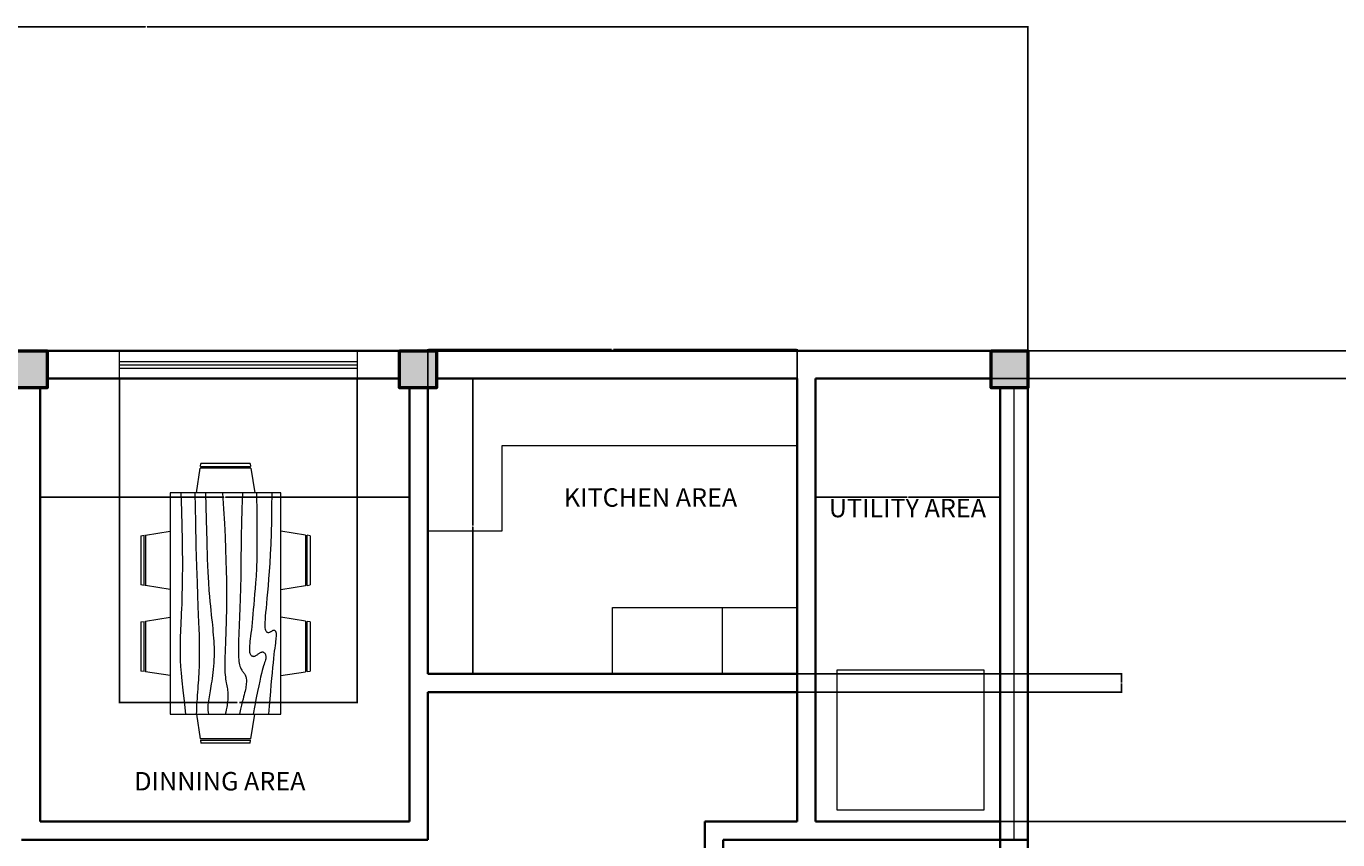
# Model space of a CAD drawing. Units: inches. Extents: x 369 to 4994, y 516 to 1297.
# Tile 3 of 9: x 722 to 1148, y 880 to 1144. Entities that reach past the tile are written whole.
import ezdxf

# ---------------------------------------------------------------- set-up
doc = ezdxf.new("R2010")
doc.units = ezdxf.units.IN
doc.header["$MEASUREMENT"] = 0
for name, color, linetype, lineweight in [('A-ANNO-DIMS', 2, 'Continuous', 18), ('A-AREA-IDEN', 7, 'Continuous', 18), ('A-COLS', 7, 'Continuous', 50), ('A-FLOR-CASE', 8, 'Continuous', 18), ('A-FURN', 8, 'Continuous', 18), ('A-GLAZ', 4, 'Continuous', 18), ('A-WALL', 7, 'Continuous', 35)]:
    doc.layers.add(name, color=color, linetype=linetype, lineweight=lineweight)
doc.layers.add('A-COLS-PATT', color=18, linetype='Continuous', lineweight=13, true_color=0x000000)
doc.styles.get("Standard").update_dxf_attribs({"font": 'arial.ttf'})
doc.dimstyles.get("Standard").update_dxf_attribs({"dimtxt": 0.18, "dimasz": 0.18, "dimexe": 0.18, "dimexo": 0.0625, "dimgap": 0.09, "dimtad": 0, "dimtih": 1, "dimtoh": 1, "dimdec": 4, "dimzin": 0, "dimdsep": 46, "dimtxsty": 'Standard', "dimcen": 0.09, "dimadec": 0, "dimazin": 0, "dimtfac": 1, "dimtdec": 4, "dimtofl": 0, "dimtmove": 0, "dimatfit": 3, "dimfxl": 1, "dimtolj": 1, "dimtzin": 0, "dimarcsym": 0})

# ---------------------------------------------------------------- blocks, each defined once
blk = doc.blocks.new('Dining Set - 36 x 72 in.')
for p, q in [((-22.2343, 26.00059), (-23.4847, 17.99762)), ((-22.2304, 26), (-5.7608, 26)), ((-22, 27.5), (-22.1562, 26.50042)), ((-5.8416, 26.5), (-22.1534, 26.5)), ((-22, 27.5), (-6, 27.5)), ((-5.8437, 26.49966), (-6, 27.5)), ((-4.5152, 17.99762), (-5.7655, 25.99926)), ((5.7657, 26.00059), (4.5153, 17.99762)), ((5.7696, 26), (22.2392, 26)), ((6, 27.5), (5.8438, 26.50042)), ((22.1584, 26.5), (5.8466, 26.5)), ((6, 27.5), (22, 27.5)), ((22.1563, 26.49966), (22, 27.5)), ((23.4848, 17.99762), (22.2345, 25.99926)), ((36, 18), (-36, 18)), ((-36, 18), (-36, -18)), ((36, -18), (36, 18)), ((-44.0006, 8.23428), (-35.9976, 9.48474)), ((44.0006, 8.23428), (35.9976, 9.48474)), ((-45.5, 8), (-44.5004, 8.15617)), ((-45.5, 8), (-45.5, -8)), ((-44.5, -8.15843), (-44.5, 8.15338)), ((-44, 8.23041), (-44, -8.23915)), ((44, 8.23041), (44, -8.23915)), ((44.5, -8.15843), (44.5, 8.15338)), ((45.5, 8), (44.5005, 8.15617)), ((45.5, 8), (45.5, -8)), ((-44.4997, -8.15631), (-45.5, -8)), ((-35.9976, -9.48476), (-43.9993, -8.2345)), ((35.9976, -9.48476), (43.9993, -8.2345)), ((44.4997, -8.15631), (45.5, -8)), ((-36, -18), (36, -18)), ((-22.2343, -26.0006), (-23.4847, -17.99762)), ((-4.5152, -17.99762), (-5.7655, -25.99928)), ((5.7657, -26.0006), (4.5153, -17.99762)), ((23.4848, -17.99762), (22.2345, -25.99928)), ((-22.2304, -26), (-5.7608, -26)), ((-22, -27.5), (-22.1562, -26.50044)), ((-5.8416, -26.5), (-22.1534, -26.5)), ((-22, -27.5), (-6, -27.5)), ((-5.8437, -26.49967), (-6, -27.5)), ((5.7696, -26), (22.2392, -26)), ((6, -27.5), (5.8438, -26.50044)), ((22.1584, -26.5), (5.8466, -26.5)), ((6, -27.5), (22, -27.5)), ((22.1563, -26.49967), (22, -27.5))]:
    blk.add_line(p, q)
for points in [[(-36, 15), (-31.1772, 14.97754), (-26.8079, 14.91406), (-22.8538, 14.81543), (-19.276, 14.6875), (-16.0362, 14.53613), (-13.0957, 14.36718), (-10.4159, 14.18652), (-7.9583, 14), (-5.6904, 13.81315), (-3.6035, 13.63021), (-1.6954, 13.45508), (0.0365, 13.29166), (1.5945, 13.14388), (2.9811, 13.01562), (4.1988, 12.9108), (5.25, 12.83333), (6.1393, 12.78613), (6.8802, 12.76823), (7.4883, 12.77767), (7.9792, 12.8125), (8.3685, 12.87077), (8.6719, 12.95052), (8.9049, 13.0498), (9.0833, 13.16666), (9.2205, 13.29899), (9.3216, 13.44401), (9.3895, 13.59879), (9.4271, 13.76041), (9.4373, 13.92594), (9.4232, 14.09245), (9.3875, 14.257), (9.3333, 14.41666), (9.2638, 14.56917), (9.1836, 14.71484), (9.0975, 14.85465), (9.0104, 14.98958), (8.9272, 15.1206), (8.8529, 15.2487), (8.7922, 15.37483), (8.75, 15.5), (8.7305, 15.62467), (8.7344, 15.74739), (8.7617, 15.86621), (8.8125, 15.97916), (8.8867, 16.08431), (8.9844, 16.17968), (9.1055, 16.26334), (9.25, 16.33333), (9.4189, 16.38802), (9.6172, 16.42708), (9.8506, 16.45052), (10.125, 16.45833), (10.4463, 16.45052), (10.8203, 16.42708), (11.2529, 16.38802), (11.75, 16.33333), (12.3184, 16.26318), (12.9694, 16.17838), (13.7151, 16.07991), (14.5677, 15.96875), (15.5395, 15.84586), (16.6426, 15.71224), (17.8893, 15.56884), (19.2917, 15.41666), (20.859, 15.25667), (22.5879, 15.08984), (24.4721, 14.91715), (26.5052, 14.73958), (28.6809, 14.5581), (30.9929, 14.3737), (33.4347, 14.18733), (36, 14)], [(-36, 10), (-28.9766, 10.14274), (-23.1725, 10.20442), (-18.4241, 10.19775), (-14.5677, 10.13541), (-11.4399, 10.03011), (-8.877, 9.89453), (-6.7154, 9.74137), (-4.7917, 9.58333), (-2.9698, 9.43082), (-1.2246, 9.28515), (0.4415, 9.14534), (2.026, 9.01041), (3.5266, 8.87939), (4.9408, 8.7513), (6.266, 8.62516), (7.5, 8.5), (8.6411, 8.37549), (9.6914, 8.2539), (10.6538, 8.13818), (11.5312, 8.03125), (12.3267, 7.93603), (13.043, 7.85547), (13.6831, 7.79248), (14.25, 7.75), (14.7471, 7.7303), (15.1797, 7.73307), (15.5537, 7.75732), (15.875, 7.80208), (16.1494, 7.86637), (16.3828, 7.94922), (16.5811, 8.04964), (16.75, 8.16666), (16.8944, 8.29915), (17.0143, 8.44531), (17.1089, 8.60319), (17.1771, 8.77083), (17.218, 8.94629), (17.2305, 9.1276), (17.2137, 9.31282), (17.1667, 9.5), (17.0895, 9.6875), (16.987, 9.875), (16.8649, 10.0625), (16.7292, 10.25), (16.5856, 10.4375), (16.4401, 10.625), (16.2985, 10.8125), (16.1667, 11), (16.05, 11.18733), (15.9518, 11.3737), (15.8752, 11.5581), (15.8229, 11.73958), (15.798, 11.91715), (15.8034, 12.08984), (15.842, 12.25667), (15.9167, 12.41666), (16.0295, 12.56836), (16.1784, 12.70833), (16.3605, 12.83268), (16.5729, 12.9375), (16.8127, 13.01888), (17.0768, 13.07291), (17.3625, 13.0957), (17.6667, 13.08333), (17.9894, 13.03312), (18.3418, 12.94726), (18.7382, 12.82918), (19.1927, 12.68229), (19.7195, 12.51001), (20.3327, 12.31575), (21.0465, 12.10294), (21.875, 11.875), (22.8357, 11.63354), (23.959, 11.37304), (25.2786, 11.08618), (26.8282, 10.76562), (28.6414, 10.40405), (30.752, 9.99414), (33.1936, 9.52856), (36, 9)], [(-36, 5.5), (-30.7157, 5.3348), (-26.069, 5.20963), (-21.9946, 5.11767), (-18.4271, 5.05208), (-15.3009, 5.00602), (-12.5508, 4.97265), (-10.1112, 4.94515), (-7.9167, 4.91666), (-5.909, 4.88167), (-4.0586, 4.83984), (-2.3429, 4.79215), (-0.7396, 4.73958), (0.7739, 4.6831), (2.22, 4.6237), (3.6213, 4.56233), (5, 4.5), (6.373, 4.43782), (7.7344, 4.3776), (9.0723, 4.32129), (10.375, 4.27083), (11.6309, 4.22819), (12.8281, 4.19531), (13.9551, 4.17415), (15, 4.16666), (15.954, 4.17448), (16.819, 4.19791), (17.6001, 4.23698), (18.3021, 4.29166), (18.9299, 4.36198), (19.4883, 4.44791), (19.9823, 4.54948), (20.4167, 4.66666), (20.7969, 4.79899), (21.1302, 4.94401), (21.4245, 5.09879), (21.6875, 5.26041), (21.9271, 5.42594), (22.1511, 5.59245), (22.3672, 5.757), (22.5834, 5.91666), (22.8065, 6.06868), (23.0404, 6.21093), (23.2879, 6.34147), (23.5521, 6.45833), (23.8358, 6.55957), (24.142, 6.64323), (24.4735, 6.70735), (24.8334, 6.75), (25.2235, 6.76969), (25.642, 6.76692), (26.0858, 6.74267), (26.5521, 6.69791), (27.0379, 6.63362), (27.5404, 6.55078), (28.0565, 6.45036), (28.5834, 6.33333), (29.1242, 6.19987), (29.7071, 6.04687), (30.3661, 5.87044), (31.1354, 5.66666), (32.0493, 5.43164), (33.142, 5.16146), (34.4475, 4.85221), (36, 4.5)], [(-36, -1), (-30.7915, -0.6591), (-26.0195, -0.38216), (-21.6519, -0.16284), (-17.6563, 0.00521), (-14.0005, 0.12833), (-10.6523, 0.21289), (-7.5796, 0.26522), (-4.75, 0.29166), (-2.134, 0.29793), (0.2878, 0.28711), (2.5317, 0.26163), (4.6146, 0.22396), (6.5529, 0.17651), (8.3633, 0.12174), (10.0623, 0.06209), (11.6667, 0), (13.1899, -0.06201), (14.6341, -0.1211), (15.9982, -0.17432), (17.2813, -0.21875), (18.4823, -0.25147), (19.6003, -0.26953), (20.6343, -0.27002), (21.5834, -0.25), (22.4481, -0.20768), (23.2357, -0.14584), (23.9549, -0.06836), (24.6146, 0.02083), (25.2235, 0.11784), (25.7904, 0.21875), (26.3241, 0.31966), (26.8334, 0.41666), (27.3265, 0.50618), (27.8099, 0.58593), (28.2894, 0.65397), (28.7709, 0.70833), (29.2601, 0.74707), (29.763, 0.76823), (30.2855, 0.76985), (30.8334, 0.75), (31.4088, 0.70784), (31.9994, 0.64713), (32.589, 0.57275), (33.1615, 0.48958), (33.7008, 0.4025), (34.1908, 0.3164), (34.6153, 0.23616), (34.9584, 0.16666), (35.2099, 0.11165), (35.3848, 0.07031), (35.504, 0.04069), (35.5886, 0.02083), (35.6594, 0.00879), (35.7377, 0.0026), (35.8442, 0.00032), (36, 0)], [(-36, -6.5), (-27.1843, -6.31267), (-20.084, -6.1263), (-14.469, -5.9419), (-10.1094, -5.76042), (-6.7752, -5.58285), (-4.2363, -5.41016), (-2.2629, -5.24333), (-0.625, -5.08334), (0.8708, -4.93099), (2.2715, -4.78646), (3.5872, -4.64974), (4.8281, -4.52084), (6.0046, -4.39974), (7.127, -4.28646), (8.2053, -4.18099), (9.25, -4.08334), (10.2705, -3.99382), (11.2734, -3.91407), (12.2647, -3.84603), (13.25, -3.79167), (14.2354, -3.75293), (15.2266, -3.73177), (16.2295, -3.73015), (17.25, -3.75), (18.2912, -3.79248), (19.3451, -3.85547), (20.4009, -3.93604), (21.4479, -4.03125), (22.4754, -4.13819), (23.4727, -4.25391), (24.4289, -4.37549), (25.3334, -4.5), (26.1785, -4.62492), (26.9694, -4.74935), (27.7145, -4.87281), (28.4219, -4.99479), (29.1, -5.11483), (29.7572, -5.23242), (30.4016, -5.34709), (31.0417, -5.45834), (31.6837, -5.56437), (32.3262, -5.65821), (32.9658, -5.73153), (33.599, -5.77604), (34.2224, -5.78345), (34.8327, -5.74545), (35.4264, -5.65373), (36, -5.5)], [(-36, -10), (-26.4022, -9.81299), (-18.4675, -9.62891), (-11.9839, -9.45069), (-6.7396, -9.28125), (-2.5226, -9.12354), (0.8789, -8.98047), (3.6769, -8.85498), (6.0833, -8.75), (8.2767, -8.66765), (10.3021, -8.60677), (12.1712, -8.56543), (13.8958, -8.54167), (15.4876, -8.53353), (16.9583, -8.53907), (18.3197, -8.55632), (19.5834, -8.58334), (20.7616, -8.61841), (21.8685, -8.66081), (22.9188, -8.71004), (23.9271, -8.76563), (24.9081, -8.82707), (25.8763, -8.89388), (26.8465, -8.96558), (27.8334, -9.04167), (28.8474, -9.12118), (29.8828, -9.20117), (30.93, -9.27824), (31.9792, -9.34896), (33.0205, -9.40991), (34.0443, -9.45768), (35.0407, -9.48885), (36, -9.5)], [(-36, -14.5), (-30.0881, -14.33513), (-25.0332, -14.21224), (-20.7312, -14.12647), (-17.0781, -14.07292), (-13.97, -14.04671), (-11.3027, -14.04297), (-8.9724, -14.05681), (-6.875, -14.08334), (-4.9224, -14.11833), (-3.0905, -14.16016), (-1.3709, -14.20785), (0.2448, -14.26042), (1.7647, -14.3169), (3.1973, -14.3763), (4.5507, -14.43767), (5.8333, -14.5), (7.0554, -14.5621), (8.235, -14.62175), (9.3922, -14.67652), (10.5469, -14.72396), (11.7192, -14.76164), (12.929, -14.78711), (14.1965, -14.79794), (15.5417, -14.79167), (16.9933, -14.76424), (18.6152, -14.70508), (20.4804, -14.60197), (22.6615, -14.44271), (25.2312, -14.21509), (28.2624, -13.9069), (31.8277, -13.50594), (36, -13)]]:
    blk.add_lwpolyline(points)
blk = doc.blocks.new('*D39')
at = {"layer": 'A-ANNO-DIMS', "color": 0, "lineweight": -2, "transparency": 16777216}
for p, q in [((474.26, 1038.85), (474.26, 1144.37)), ((474.44, 1144.19), (760.47, 1144.19)), ((1047.08, 1144.19), (761.05, 1144.19)), ((1047.26, 1038.85), (1047.26, 1144.37))]:
    blk.add_line(p, q, dxfattribs=at)
at = {"layer": 'A-ANNO-DIMS', "color": 0, "transparency": 16777216}
for points in [[(474.44, 1144.22), (474.44, 1144.16), (474.26, 1144.19)], [(1047.08, 1144.22), (1047.08, 1144.16), (1047.26, 1144.19)]]:
    blk.add_solid(points, dxfattribs=at)
at = {"layer": 'Defpoints', "color": 0, "transparency": 16777216}
for p in [(1047.26, 1144.19), (474.26, 1038.79), (1047.26, 1038.79)]:
    blk.add_point(p, dxfattribs=at)
at = {"layer": 'A-ANNO-DIMS', "color": 0, "transparency": 16777216, "insert": (760.76, 1144.19), "char_height": 0.18, "attachment_point": 5}
blk.add_mtext('\\A1;573', dxfattribs=at)
blk = doc.blocks.new('*D43')
at = {"layer": 'A-ANNO-DIMS', "color": 0, "lineweight": -2, "transparency": 16777216}
for p, q in [((726.26, 885.85), (726.26, 991.37)), ((726.44, 991.19), (785.98, 991.19)), ((846.08, 991.19), (786.54, 991.19)), ((846.26, 885.85), (846.26, 991.37))]:
    blk.add_line(p, q, dxfattribs=at)
at = {"layer": 'A-ANNO-DIMS', "color": 0, "transparency": 16777216}
for points in [[(726.44, 991.22), (726.44, 991.16), (726.26, 991.19)], [(846.08, 991.22), (846.08, 991.16), (846.26, 991.19)]]:
    blk.add_solid(points, dxfattribs=at)
at = {"layer": 'Defpoints', "color": 0, "transparency": 16777216}
for p in [(846.26, 991.19), (726.26, 885.79), (846.26, 885.79)]:
    blk.add_point(p, dxfattribs=at)
at = {"layer": 'A-ANNO-DIMS', "color": 0, "transparency": 16777216, "insert": (786.26, 991.19), "char_height": 0.18, "attachment_point": 5}
blk.add_mtext('\\A1;120', dxfattribs=at)
blk = doc.blocks.new('*D44')
at = {"layer": 'A-ANNO-DIMS', "color": 0, "lineweight": -2, "transparency": 16777216}
for p, q in [((852.26, 933.85), (852.26, 1039.37)), ((852.44, 1039.19), (911.98, 1039.19)), ((972.08, 1039.19), (912.54, 1039.19)), ((972.26, 933.85), (972.26, 1039.37))]:
    blk.add_line(p, q, dxfattribs=at)
at = {"layer": 'A-ANNO-DIMS', "color": 0, "transparency": 16777216}
for points in [[(852.44, 1039.22), (852.44, 1039.16), (852.26, 1039.19)], [(972.08, 1039.22), (972.08, 1039.16), (972.26, 1039.19)]]:
    blk.add_solid(points, dxfattribs=at)
at = {"layer": 'Defpoints', "color": 0, "transparency": 16777216}
for p in [(972.26, 1039.19), (852.26, 933.79), (972.26, 933.79)]:
    blk.add_point(p, dxfattribs=at)
at = {"layer": 'A-ANNO-DIMS', "color": 0, "transparency": 16777216, "insert": (912.26, 1039.19), "char_height": 0.18, "attachment_point": 5}
blk.add_mtext('\\A1;120', dxfattribs=at)
blk = doc.blocks.new('*D45')
at = {"layer": 'A-ANNO-DIMS', "color": 0, "lineweight": -2, "transparency": 16777216}
for p, q in [((978.26, 885.85), (978.26, 991.37)), ((978.44, 991.19), (1008.04, 991.19)), ((1038.08, 991.19), (1008.48, 991.19)), ((1038.26, 885.85), (1038.26, 991.37))]:
    blk.add_line(p, q, dxfattribs=at)
at = {"layer": 'A-ANNO-DIMS', "color": 0, "transparency": 16777216}
for points in [[(978.44, 991.22), (978.44, 991.16), (978.26, 991.19)], [(1038.08, 991.22), (1038.08, 991.16), (1038.26, 991.19)]]:
    blk.add_solid(points, dxfattribs=at)
at = {"layer": 'Defpoints', "color": 0, "transparency": 16777216}
for p in [(1038.26, 991.19), (978.26, 885.79), (1038.26, 885.79)]:
    blk.add_point(p, dxfattribs=at)
at = {"layer": 'A-ANNO-DIMS', "color": 0, "transparency": 16777216, "insert": (1008.26, 991.19), "char_height": 0.18, "attachment_point": 5}
blk.add_mtext('\\A1;60', dxfattribs=at)
blk = doc.blocks.new('*D46')
at = {"layer": 'A-ANNO-DIMS', "color": 0, "lineweight": -2, "transparency": 16777216}
for p, q in [((978.32, 1029.79), (2671.51, 1029.79)), ((2671.33, 1029.61), (2671.33, 957.97)), ((2671.33, 885.97), (2671.33, 957.61)), ((1038.32, 885.79), (2671.51, 885.79))]:
    blk.add_line(p, q, dxfattribs=at)
at = {"layer": 'A-ANNO-DIMS', "color": 0, "transparency": 16777216}
for points in [[(2671.3, 1029.61), (2671.36, 1029.61), (2671.33, 1029.79)], [(2671.3, 885.97), (2671.36, 885.97), (2671.33, 885.79)]]:
    blk.add_solid(points, dxfattribs=at)
at = {"layer": 'Defpoints', "color": 0, "transparency": 16777216}
for p in [(978.26, 1029.79), (2671.33, 1029.79), (1038.26, 885.79)]:
    blk.add_point(p, dxfattribs=at)
at = {"layer": 'A-ANNO-DIMS', "color": 0, "transparency": 16777216, "insert": (2671.33, 957.79), "char_height": 0.18, "attachment_point": 5}
blk.add_mtext('\\A1;144', dxfattribs=at)
blk = doc.blocks.new('*D54')
at = {"layer": 'A-ANNO-DIMS', "color": 0, "lineweight": -2, "transparency": 16777216}
for p, q in [((972.2, 1029.79), (866.68, 1029.79)), ((866.86, 1029.61), (866.86, 981.97)), ((866.86, 933.97), (866.86, 981.61)), ((972.2, 933.79), (866.68, 933.79))]:
    blk.add_line(p, q, dxfattribs=at)
at = {"layer": 'A-ANNO-DIMS', "color": 0, "transparency": 16777216}
for points in [[(866.83, 1029.61), (866.89, 1029.61), (866.86, 1029.79)], [(866.83, 933.97), (866.89, 933.97), (866.86, 933.79)]]:
    blk.add_solid(points, dxfattribs=at)
at = {"layer": 'Defpoints', "color": 0, "transparency": 16777216}
for p in [(866.86, 1029.79), (972.26, 1029.79), (972.26, 933.79)]:
    blk.add_point(p, dxfattribs=at)
at = {"layer": 'A-ANNO-DIMS', "color": 0, "transparency": 16777216, "insert": (866.86, 981.79), "char_height": 0.18, "attachment_point": 5}
blk.add_mtext('\\A1;96', dxfattribs=at)
blk = doc.blocks.new('*D65')
at = {"layer": 'A-ANNO-DIMS', "color": 0, "lineweight": -2, "transparency": 16777216}
for p, q in [((752.08, 1029.73), (752.08, 924.21)), ((829.25, 1029.73), (829.25, 924.21)), ((752.26, 924.39), (790.27, 924.39)), ((829.07, 924.39), (791.06, 924.39))]:
    blk.add_line(p, q, dxfattribs=at)
at = {"layer": 'A-ANNO-DIMS', "color": 0, "transparency": 16777216}
for points in [[(752.26, 924.42), (752.26, 924.36), (752.08, 924.39)], [(829.07, 924.42), (829.07, 924.36), (829.25, 924.39)]]:
    blk.add_solid(points, dxfattribs=at)
at = {"layer": 'Defpoints', "color": 0, "transparency": 16777216}
for p in [(752.08, 1029.79), (829.25, 1029.79), (752.08, 924.39)]:
    blk.add_point(p, dxfattribs=at)
at = {"layer": 'A-ANNO-DIMS', "color": 0, "transparency": 16777216, "insert": (790.66, 924.39), "char_height": 0.18, "attachment_point": 5}
blk.add_mtext('\\A1;77.17', dxfattribs=at)
blk = doc.blocks.new('*D72')
at = {"layer": 'A-ANNO-DIMS', "color": 0, "lineweight": -2, "transparency": 16777216}
for p, q in [((972.32, 933.79), (1077.84, 933.79)), ((1077.66, 933.61), (1077.66, 930.97)), ((1077.66, 927.97), (1077.66, 930.61)), ((972.32, 927.79), (1077.84, 927.79))]:
    blk.add_line(p, q, dxfattribs=at)
at = {"layer": 'A-ANNO-DIMS', "color": 0, "transparency": 16777216}
for points in [[(1077.63, 933.61), (1077.69, 933.61), (1077.66, 933.79)], [(1077.63, 927.97), (1077.69, 927.97), (1077.66, 927.79)]]:
    blk.add_solid(points, dxfattribs=at)
at = {"layer": 'Defpoints', "color": 0, "transparency": 16777216}
for p in [(972.26, 933.79), (972.26, 927.79), (1077.66, 927.79)]:
    blk.add_point(p, dxfattribs=at)
at = {"layer": 'A-ANNO-DIMS', "color": 0, "transparency": 16777216, "insert": (1077.66, 930.79), "char_height": 0.18, "attachment_point": 5}
blk.add_mtext('\\A1;6', dxfattribs=at)
blk = doc.blocks.new('*D75')
at = {"layer": 'A-ANNO-DIMS', "color": 0, "lineweight": -2, "transparency": 16777216}
for p, q in [((1208.31, 1038.79), (368.68, 1038.79)), ((368.86, 1038.61), (368.86, 830.47)), ((368.86, 621.97), (368.86, 830.11)), ((1262.31, 621.79), (368.68, 621.79))]:
    blk.add_line(p, q, dxfattribs=at)
at = {"layer": 'A-ANNO-DIMS', "color": 0, "transparency": 16777216}
for points in [[(368.83, 1038.61), (368.89, 1038.61), (368.86, 1038.79)], [(368.83, 621.97), (368.89, 621.97), (368.86, 621.79)]]:
    blk.add_solid(points, dxfattribs=at)
at = {"layer": 'Defpoints', "color": 0, "transparency": 16777216}
for p in [(368.86, 1038.79), (1208.37, 1038.79), (1262.37, 621.79)]:
    blk.add_point(p, dxfattribs=at)
at = {"layer": 'A-ANNO-DIMS', "color": 0, "transparency": 16777216, "insert": (368.86, 830.29), "char_height": 0.18, "attachment_point": 5}
blk.add_mtext('\\A1;417', dxfattribs=at)
blk = doc.blocks.new('*D98')
at = {"layer": 'A-ANNO-DIMS', "color": 0, "lineweight": -2, "transparency": 16777216}
for p, q in [((1992.86, 1038.79), (368.68, 1038.79)), ((368.86, 1038.61), (368.86, 830.47)), ((368.86, 621.97), (368.86, 830.11)), ((2046.86, 621.79), (368.68, 621.79))]:
    blk.add_line(p, q, dxfattribs=at)
at = {"layer": 'A-ANNO-DIMS', "color": 0, "transparency": 16777216}
for points in [[(368.83, 1038.61), (368.89, 1038.61), (368.86, 1038.79)], [(368.83, 621.97), (368.89, 621.97), (368.86, 621.79)]]:
    blk.add_solid(points, dxfattribs=at)
at = {"layer": 'Defpoints', "color": 0, "transparency": 16777216}
for p in [(368.86, 1038.79), (1992.93, 1038.79), (2046.93, 621.79)]:
    blk.add_point(p, dxfattribs=at)
at = {"layer": 'A-ANNO-DIMS', "color": 0, "transparency": 16777216, "insert": (368.86, 830.29), "char_height": 0.18, "attachment_point": 5}
blk.add_mtext('\\A1;417', dxfattribs=at)

msp = doc.modelspace()

# ---------------------------------------------------------------- hatches: boundary and pattern name
at = {"layer": 'A-COLS-PATT'}
h = msp.add_hatch(color=256, dxfattribs=at)
h.dxf.hatch_style = 1
h.paths.add_polyline_path([(540.2581, 633.7894), (528.2581, 633.7894), (528.2581, 621.7894), (540.2581, 621.7894)])
h.paths.add_polyline_path([(726.2581, 633.7894), (714.2581, 633.7894), (714.2581, 621.7894), (726.2581, 621.7894)])
h.paths.add_polyline_path([(918.2581, 633.7894), (906.2581, 633.7894), (906.2581, 621.7894), (918.2581, 621.7894)])
h.paths.add_polyline_path([(1047.2581, 633.7894), (1035.2581, 633.7894), (1035.2581, 621.7894), (1047.2581, 621.7894)])
h.paths.add_polyline_path([(1047.2581, 798.6977), (1035.2581, 798.6977), (1035.2581, 786.6977), (1047.2581, 786.6977)])
h.paths.add_polyline_path([(918.2581, 795.7894), (906.2581, 795.7894), (906.2581, 783.7894), (918.2581, 783.7894)])
h.paths.add_polyline_path([(726.2581, 795.7894), (714.2581, 795.7894), (714.2581, 783.7894), (726.2581, 783.7894)])
h.paths.add_polyline_path([(1047.2581, 1038.7894), (1035.2581, 1038.7894), (1035.2581, 1026.7894), (1047.2581, 1026.7894)])
h.paths.add_polyline_path([(855.044, 1038.7894), (843.044, 1038.7894), (843.044, 1026.7894), (855.044, 1026.7894)])
h.paths.add_polyline_path([(728.5536, 1038.7894), (716.5536, 1038.7894), (716.5536, 1026.7894), (728.5536, 1026.7894)])
h.paths.add_polyline_path([(543.2581, 1038.7894), (531.2581, 1038.7894), (531.2581, 1026.7894), (543.2581, 1026.7894)])
h.paths.add_polyline_path([(543.2581, 792.9013), (531.2581, 792.9013), (531.2581, 780.9013), (543.2581, 780.9013), (543.2581, 783.7894)])
h.paths.add_polyline_path([(1274.3738, 633.7894), (1262.3738, 633.7894), (1262.3738, 621.7894), (1274.3738, 621.7894)])
h.paths.add_polyline_path([(1460.3738, 633.7894), (1448.3738, 633.7894), (1448.3738, 621.7894), (1460.3738, 621.7894)])
h.paths.add_polyline_path([(1652.3738, 633.7894), (1640.3738, 633.7894), (1640.3738, 621.7894), (1652.3738, 621.7894)])
h.paths.add_polyline_path([(1781.3738, 633.7894), (1769.3738, 633.7894), (1769.3738, 621.7894), (1781.3738, 621.7894)])
h.paths.add_polyline_path([(1781.3738, 1038.7894), (1769.3738, 1038.7894), (1769.3738, 1026.7894), (1781.3738, 1026.7894)])
h.paths.add_polyline_path([(1625.484, 1038.7894), (1613.484, 1038.7894), (1613.484, 1026.7894), (1615.6962, 1026.7894), (1625.484, 1026.7894)])
h.paths.add_polyline_path([(1462.6692, 1038.7894), (1450.6692, 1038.7894), (1450.6692, 1026.7894), (1462.6692, 1026.7894)])
h.paths.add_polyline_path([(1277.3738, 1038.7894), (1265.3738, 1038.7894), (1265.3738, 1026.7894), (1277.3738, 1026.7894)])
h.paths.add_polyline_path([(1460.3738, 807.7894), (1448.3738, 807.7894), (1448.3738, 795.7894), (1460.3738, 795.7894)])
h.paths.add_polyline_path([(1652.3738, 807.7894), (1640.3738, 807.7894), (1640.3738, 795.7894), (1652.3738, 795.7894)])
h.paths.add_polyline_path([(2244.9265, 633.7894), (2232.9265, 633.7894), (2232.9265, 621.7894), (2244.9265, 621.7894)])
h.paths.add_polyline_path([(2058.9265, 633.7894), (2046.9265, 633.7894), (2046.9265, 621.7894), (2058.9265, 621.7894)])
h.paths.add_polyline_path([(2436.9265, 633.7894), (2424.9265, 633.7894), (2424.9265, 621.7894), (2436.9265, 621.7894)])
h.paths.add_polyline_path([(2565.9265, 633.7894), (2553.9265, 633.7894), (2553.9265, 621.7894), (2565.9265, 621.7894)])
h.paths.add_polyline_path([(2565.9265, 798.6977), (2553.9265, 798.6977), (2553.9265, 786.6977), (2565.9265, 786.6977)])
h.paths.add_polyline_path([(2565.9265, 1038.7894), (2553.9265, 1038.7894), (2553.9265, 1026.7894), (2565.9265, 1026.7894)])
h.paths.add_polyline_path([(2436.9265, 1038.7894), (2424.9265, 1038.7894), (2424.9265, 1026.7894), (2436.9265, 1026.7894)])
h.paths.add_polyline_path([(2247.222, 1038.7894), (2235.222, 1038.7894), (2235.222, 1026.7894), (2247.222, 1026.7894)])
h.paths.add_polyline_path([(2061.9265, 1038.7894), (2049.9265, 1038.7894), (2049.9265, 1026.7894), (2061.9265, 1026.7894)])

# ---------------------------------------------------------------- linework, layer by layer
at = {"layer": 'A-COLS'}
for points in [[(716.5536, 1038.7894), (728.5536, 1038.7894), (728.5536, 1026.7894), (716.5536, 1026.7894)], [(843.044, 1038.7894), (855.044, 1038.7894), (855.044, 1026.7894), (843.044, 1026.7894)], [(1035.2581, 1038.7894), (1047.2581, 1038.7894), (1047.2581, 1026.7894), (1035.2581, 1026.7894)]]:
    msp.add_lwpolyline(points, close=True, dxfattribs=at)
at = {"layer": 'A-FLOR-CASE'}
for p, q in [((876.4278, 980.2894), (876.4278, 1008.0235)), ((876.4278, 1008.0235), (972.2581, 1008.0235)), ((852.2581, 980.2894), (876.4278, 980.2894)), ((912.2581, 933.7894), (912.2581, 955.3815)), ((912.2581, 955.3815), (972.2581, 955.3815)), ((948.0029, 933.7894), (948.0029, 955.3815)), ((1033.0053, 934.9372), (985.2066, 934.9372)), ((985.2066, 934.9372), (985.2066, 889.5062)), ((1033.0053, 889.5062), (1033.0053, 934.9372)), ((985.2066, 889.5062), (1033.0053, 889.5062))]:
    msp.add_line(p, q, dxfattribs=at)
at = {"layer": 'A-GLAZ'}
for p, q in [((752.0804, 1035.3655), (829.248, 1035.3655)), ((752.0804, 1034.2894), (829.248, 1034.2894)), ((752.0804, 1033.2133), (829.248, 1033.2133)), ((1042.7106, 1026.7894), (1042.7106, 879.7894))]:
    msp.add_line(p, q, dxfattribs=at)
msp.add_lwpolyline([(752.0804, 1038.7894), (829.248, 1038.7894), (829.248, 1029.7894), (752.0804, 1029.7894)], close=True, dxfattribs=at)
at = {"layer": 'A-WALL'}
for p, q in [((1038.2581, 1038.7894), (531.2581, 1038.7894)), ((843.044, 1029.7894), (728.5536, 1029.7894)), ((972.2581, 1029.7894), (855.044, 1029.7894)), ((972.2581, 1029.7894), (972.2581, 885.7894)), ((1035.2581, 1029.7894), (978.2581, 1029.7894)), ((978.2581, 1029.7894), (978.2581, 885.7894)), ((1047.2581, 621.7894), (1047.2581, 1029.7894)), ((726.2581, 1026.7894), (726.2581, 885.7894)), ((846.2581, 1026.7894), (846.2581, 933.7894)), ((852.2581, 1026.7894), (852.2581, 933.7894)), ((1038.2581, 879.7894), (1038.2581, 1026.7894)), ((846.2581, 885.7894), (846.2581, 933.7894)), ((852.2581, 933.7894), (972.2581, 933.7894)), ((852.2581, 927.7894), (972.2581, 927.7894)), ((852.2581, 927.7894), (852.2581, 879.7894)), ((726.2581, 885.7894), (846.2581, 885.7894)), ((942.2581, 885.7894), (942.2581, 788.8925)), ((972.2581, 885.7894), (942.2581, 885.7894)), ((1038.2581, 885.7894), (978.2581, 885.7894)), ((720.2581, 879.7894), (852.2581, 879.7894)), ((1047.2581, 879.7894), (948.2581, 879.7894)), ((948.2581, 879.7894), (948.2581, 794.8925)), ((1038.2581, 798.6977), (1038.2581, 879.7894))]:
    msp.add_line(p, q, dxfattribs=at)

# ---------------------------------------------------------------- block references
at = {"layer": 'A-FURN', "rotation": 270}
msp.add_blockref('Dining Set - 36 x 72 in.', (786.5308, 956.6695), dxfattribs=at)

# ---------------------------------------------------------------- texts
at = {"layer": 'A-AREA-IDEN'}
for s, p in [('KITCHEN AREA', (896.4611, 988.1046)), ('UTILITY AREA', (982.5446, 984.6655)), ('DINNING AREA', (756.8706, 895.8342))]:
    msp.add_text(s, height=6, dxfattribs=at).set_placement(p)

# ---------------------------------------------------------------- dimensions: what is measured, and where the dimension line sits
at = {"layer": 'A-ANNO-DIMS'}
for base, p1, p2, picture, middle in [((1047.2581, 1144.1894), (474.2581, 1038.7894), (1047.2581, 1038.7894), '*D39', (760.7581, 1144.1894)), ((972.2581, 1039.1894), (852.2581, 933.7894), (972.2581, 933.7894), '*D44', (912.2581, 1039.1894)), ((846.2581, 991.1894), (726.2581, 885.7894), (846.2581, 885.7894), '*D43', (786.2581, 991.1894)), ((1038.2581, 991.1894), (978.2581, 885.7894), (1038.2581, 885.7894), '*D45', (1008.2581, 991.1894))]:
    dim = msp.add_linear_dim(base=base, p1=p1, p2=p2, dimstyle='Standard', override={"dimdec": 0, "dimlfac": 1, "dimrnd": 0, "dimzin": 0, "dimdsep": 46, "dimlunit": 2}, dxfattribs=at)
    dim.commit()
    dim.dimension.update_dxf_attribs({"geometry": picture, "text_midpoint": middle})
for base, p1, p2, angle, override, picture, middle in [((368.8581, 1038.7894), (1262.3738, 621.7894), (1208.3738, 1038.7894), 90, {"dimdec": 0, "dimlfac": 1, "dimrnd": 0, "dimzin": 0, "dimdsep": 46, "dimlunit": 2}, '*D75', (368.8581, 830.2894)), ((368.8581, 1038.7894), (2046.9265, 621.7894), (1992.9265, 1038.7894), 90, {"dimdec": 0, "dimlfac": 1, "dimrnd": 0, "dimzin": 0, "dimdsep": 46, "dimlunit": 2}, '*D98', (368.8581, 830.2894)), ((752.0804, 924.3894), (829.248, 1029.7894), (752.0804, 1029.7894), 180, {"dimdec": 2, "dimlfac": 1, "dimrnd": 0, "dimzin": 0, "dimdsep": 46, "dimlunit": 2}, '*D65', (790.6642, 924.3894)), ((866.8581, 1029.7894), (972.2581, 933.7894), (972.2581, 1029.7894), 90, {"dimdec": 0, "dimlfac": 1, "dimrnd": 0, "dimzin": 0, "dimdsep": 46, "dimlunit": 2}, '*D54', (866.8581, 981.7894)), ((2671.3265, 1029.7894), (1038.2581, 885.7894), (978.2581, 1029.7894), 90, {"dimdec": 0, "dimlfac": 1, "dimrnd": 0, "dimzin": 0, "dimdsep": 46, "dimlunit": 2}, '*D46', (2671.3265, 957.7894)), ((1077.6581, 927.7894), (972.2581, 933.7894), (972.2581, 927.7894), 270, {"dimdec": 0, "dimlfac": 1, "dimrnd": 0, "dimzin": 0, "dimdsep": 46, "dimlunit": 2}, '*D72', (1077.6581, 930.7894))]:
    dim = msp.add_linear_dim(base=base, p1=p1, p2=p2, angle=angle, dimstyle='Standard', override=override, dxfattribs=at)
    dim.commit()
    dim.dimension.update_dxf_attribs({"geometry": picture, "text_midpoint": middle})

doc.saveas('drawing.dxf')
